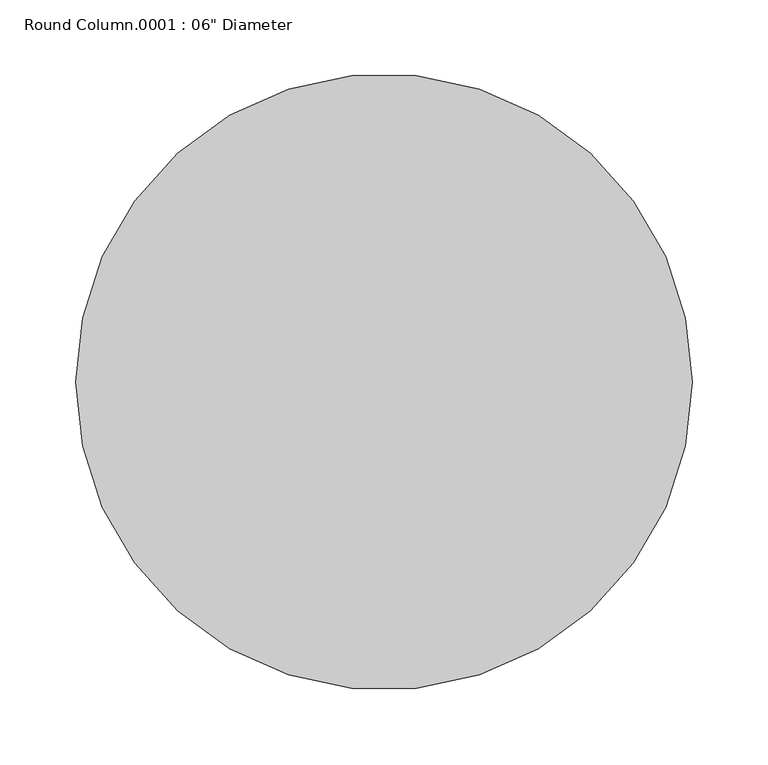
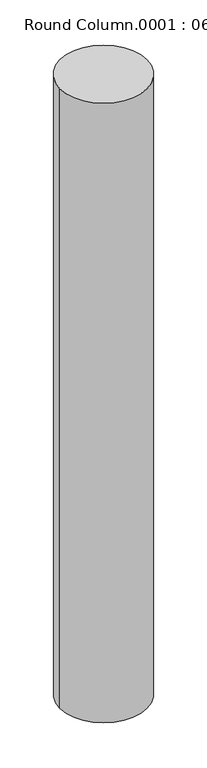
"""IFC4 building model written with IfcOpenShell, lengths in millimetres: column geometry."""

from ifc_helpers import new_model, si_unit, point, frame, frame_2d, origin, place, context, project, spatial, circle_curve, trimmed, segment, composite_curve, outline, extrude, source, transform, mapped, element, save


def column_386bdc77(model_context):
    return source(origin(), model_context, "Body", "SweptSolid", [
        extrude(outline(composite_curve([segment(trimmed(circle_curve(frame_2d((2074.9686162, 4758.9561122)), 203.2), [point((1871.7686162, 4758.9561122))], [point((2278.1686162, 4758.9561122))], False, "CARTESIAN"), True, "CONTINUOUS"), segment(trimmed(circle_curve(frame_2d((2074.9686162, 4758.9561122)), 203.2), [point((2278.1686162, 4758.9561122))], [point((1871.7686162, 4758.9561122))], False, "CARTESIAN"), True, "CONTINUOUS")], self_intersect=False)), frame((0.0, 0.0, 7010.4), z_axis=(0.0, 0.0, 1.0), x_axis=(1.0, 0.0, 0.0)), (0.0, 0.0, 1.0), 3048.0),
    ])


if __name__ == "__main__":
    model = new_model("IFC4")
    model_context = context("Model", 3, world=origin())
    ifc_project = project(units=[si_unit("LENGTHUNIT", "METRE", prefix="MILLI")], contexts=[model_context])
    site = spatial("IfcSite", under=ifc_project)
    building = spatial("IfcBuilding", under=site)
    placement = place(None, origin())
    column_shape = column_386bdc77(model_context)
    element("IfcColumn", 1, ObjectType="Round Column.0001 : 06\" Diameter", at=placement, inside=building, context=model_context, shape_type="MappedRepresentation", body=[
        mapped(column_shape, transform((0.0, 0.0, 0.0), x_axis=(1.0, 0.0, 0.0), y_axis=(0.0, 1.0, 0.0), z_axis=(0.0, 0.0, 1.0))),
    ])
    save(model, "model.ifc")

# Revit data of these elements
# Type "Round Column.0001 : 06\" Diameter"
#   Assembly Code = "B1010200"
#   Diameter = 1' - 0"
#   Offset Base = 0' - 0"
#   Offset Top = 0' - 0"
#   Material = EIFS, Exterior Insulation
# Materials
#   "EIFS, Exterior Insulation": class "Generic", colour RGB 127 127 127, transparency 0, Description = "EIFS - Exterior Insulation", Cost = 0
